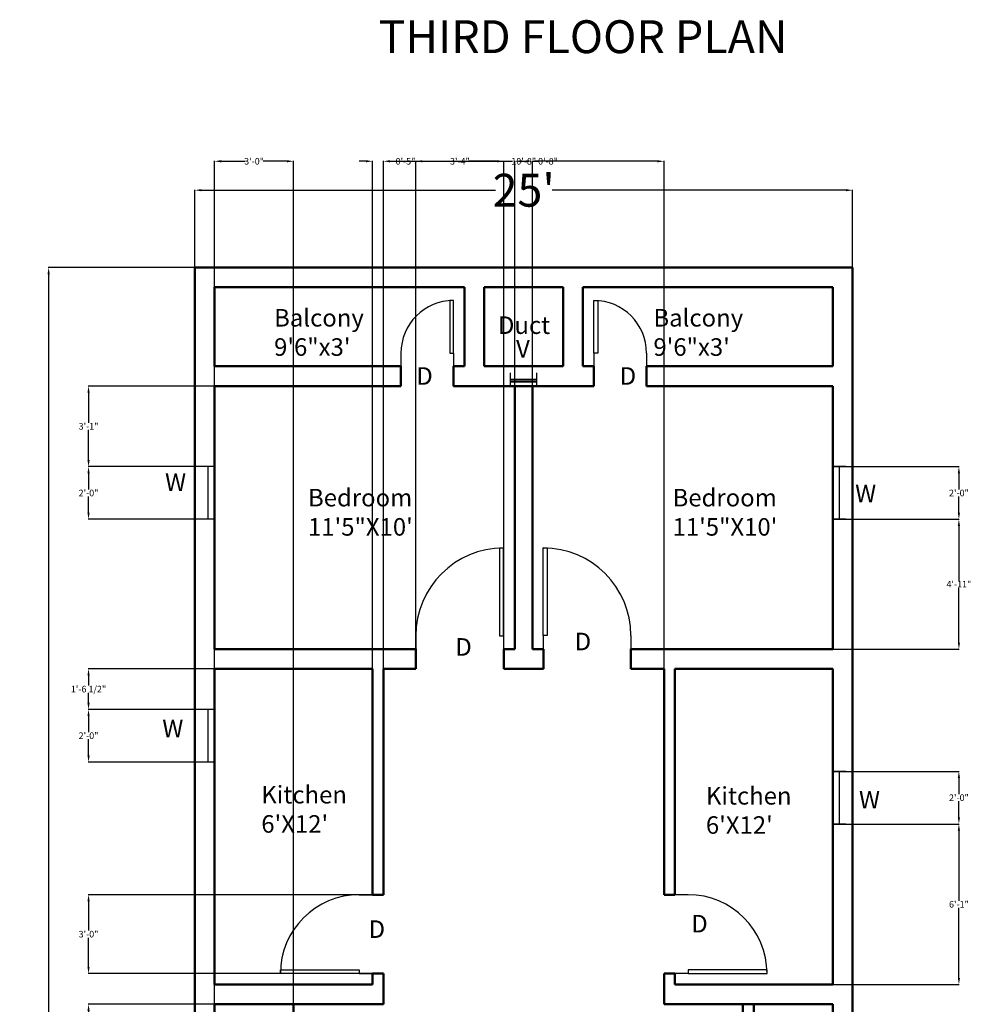
# Model space of a CAD drawing. Units: inches. Extents: x -250 to 2650, y 180 to 1183.
# Tile 8 of 10: x 1594 to 2028, y 734 to 1183. Entities that reach past the tile are written whole.
import ezdxf

# ---------------------------------------------------------------- set-up
doc = ezdxf.new("R2010")
doc.units = ezdxf.units.IN
doc.header["$MEASUREMENT"] = 0
for name, color, linetype, lineweight in [('A-ANNO-DIMS', 2, 'Continuous', 18), ('A-ANNO-TEXT', 7, 'Continuous', 18), ('A-AREA-IDEN', 3, 'Continuous', 18), ('A-DOOR', 4, 'Continuous', 25), ('A-GLAZ', 3, 'Continuous', 25), ('A-WALL', 7, 'Continuous', 50)]:
    doc.layers.add(name, color=color, linetype=linetype, lineweight=lineweight)
doc.styles.get("Standard").update_dxf_attribs({"font": 'arial.ttf'})
doc.dimstyles.get("Standard").update_dxf_attribs({"dimtxt": 3, "dimasz": 3, "dimexe": 0.18, "dimexo": 0.0625, "dimgap": 0.09, "dimtad": 0, "dimtih": 1, "dimtoh": 1, "dimdec": 0, "dimzin": 0, "dimdsep": 46, "dimlunit": 3, "dimtxsty": 'Standard', "dimcen": 0.09, "dimadec": 0, "dimazin": 0, "dimtfac": 1, "dimtdec": 0, "dimtofl": 0, "dimtmove": 0, "dimatfit": 3, "dimfxl": 1, "dimtolj": 1, "dimtzin": 0, "dimarcsym": 0})

# ---------------------------------------------------------------- blocks, each defined once
blk = doc.blocks.new('*D36')
at = {"layer": 'A-ANNO-DIMS', "color": 0, "lineweight": -2, "transparency": 16777216}
for p, q in [((1673.49, 1070.09), (1673.49, 1105.5)), ((1676.49, 1105.32), (1810.55, 1105.32)), ((1970.49, 1105.32), (1836.44, 1105.32)), ((1973.49, 1070.09), (1973.49, 1105.5))]:
    blk.add_line(p, q, dxfattribs=at)
at = {"layer": 'A-ANNO-DIMS', "color": 0, "transparency": 16777216}
for points in [[(1676.49, 1105.82), (1676.49, 1104.82), (1673.49, 1105.32)], [(1970.49, 1105.82), (1970.49, 1104.82), (1973.49, 1105.32)]]:
    blk.add_solid(points, dxfattribs=at)
at = {"layer": 'Defpoints', "color": 0, "transparency": 16777216}
for p in [(1673.49, 1105.32), (1673.49, 1070.02), (1973.49, 1070.02)]:
    blk.add_point(p, dxfattribs=at)
at = {"layer": 'A-ANNO-DIMS', "color": 0, "transparency": 16777216, "insert": (1823.49, 1105.32), "char_height": 3, "attachment_point": 5}
blk.add_mtext("\\A1;{\\H5x;25'}", dxfattribs=at)
blk = doc.blocks.new('*D37')
at = {"layer": 'A-ANNO-DIMS', "color": 0, "lineweight": -2, "transparency": 16777216}
for p, q in [((1673.43, 1070.02), (1606.61, 1070.02)), ((1606.79, 1067.02), (1606.79, 657.77)), ((1606.79, 233.02), (1606.79, 642.28)), ((1673.43, 230.02), (1606.61, 230.02))]:
    blk.add_line(p, q, dxfattribs=at)
at = {"layer": 'A-ANNO-DIMS', "color": 0, "transparency": 16777216}
for points in [[(1606.29, 1067.02), (1607.29, 1067.02), (1606.79, 1070.02)], [(1606.29, 233.02), (1607.29, 233.02), (1606.79, 230.02)]]:
    blk.add_solid(points, dxfattribs=at)
at = {"layer": 'Defpoints', "color": 0, "transparency": 16777216}
for p in [(1673.49, 1070.02), (1606.79, 230.02), (1673.49, 230.02)]:
    blk.add_point(p, dxfattribs=at)
at = {"layer": 'A-ANNO-DIMS', "color": 0, "transparency": 16777216, "insert": (1606.79, 650.02), "char_height": 3, "attachment_point": 5}
blk.add_mtext("\\A1;{\\H5x;70'}", dxfattribs=at)
blk = doc.blocks.new('*U17')
for p, q in [((-24, 0), (-24, -6)), ((0, 0), (0, -6))]:
    blk.add_line(p, q)
blk.add_lwpolyline([(0, 0), (0, 24), (-1.75, 24), (-1.75, 0)], close=True)
blk.add_arc((0, 0), 24, 90, 180)
blk = doc.blocks.new('*U18')
for p, q in [((0, 0), (0, -6)), ((24, 0), (24, -6))]:
    blk.add_line(p, q)
blk.add_lwpolyline([(0, 0), (0, 24), (1.75, 24), (1.75, 0)], close=True)
blk.add_arc((0, 0), 24, 0, 90)
blk = doc.blocks.new('*U24')
for p, q in [((-24, 6), (-24, 0)), ((0, 6), (0, 0)), ((0, 3), (-24, 3))]:
    blk.add_line(p, q)
blk = doc.blocks.new('*U23')
for p, q in [((-24, 6), (-24, 0)), ((0, 6), (0, 0)), ((0, 3), (-24, 3))]:
    blk.add_line(p, q)
blk = doc.blocks.new('*U40')
for p, q in [((0, 0), (0, -6)), ((40, 0), (40, -6))]:
    blk.add_line(p, q)
blk.add_lwpolyline([(0, 0), (0, 40), (1.75, 40), (1.75, 0)], close=True)
blk.add_arc((0, 0), 40, 0, 90)
blk = doc.blocks.new('*U41')
for p, q in [((0, 0), (0, -6)), ((-40, 0), (-40, -6))]:
    blk.add_line(p, q)
blk.add_lwpolyline([(0, 0), (0, 40), (-1.75, 40), (-1.75, 0)], close=True)
blk.add_arc((0, 0), 40, 90, 180)
blk = doc.blocks.new('*U42')
for p, q in [((0, 0), (0, -6)), ((-36, 0), (-36, -6))]:
    blk.add_line(p, q)
blk.add_lwpolyline([(0, 0), (0, 36), (-1.75, 36), (-1.75, 0)], close=True)
blk.add_arc((0, 0), 36, 90, 180)
blk = doc.blocks.new('*U43')
for p, q in [((-36, 0), (-36, 6)), ((0, 0), (0, 6))]:
    blk.add_line(p, q)
blk.add_lwpolyline([(0, 0), (0, -36), (-1.75, -36), (-1.75, 0)], close=True)
blk.add_arc((0, 0), 36, 180, 270)
blk = doc.blocks.new('*U22')
for p, q in [((0, 6), (0, 0)), ((12, 6), (12, 0)), ((0, 3), (12, 3))]:
    blk.add_line(p, q)
blk = doc.blocks.new('*D143')
at = {"layer": 'A-ANNO-DIMS', "color": 0, "lineweight": -2, "transparency": 16777216}
for p, q in [((1682.49, 734.09), (1682.49, 1118.7)), ((1685.49, 1118.52), (1696.42, 1118.52)), ((1715.49, 1118.52), (1704.57, 1118.52)), ((1718.49, 734.09), (1718.49, 1118.7))]:
    blk.add_line(p, q, dxfattribs=at)
at = {"layer": 'A-ANNO-DIMS', "color": 0, "transparency": 16777216}
for points in [[(1685.49, 1119.02), (1685.49, 1118.02), (1682.49, 1118.52)], [(1715.49, 1119.02), (1715.49, 1118.02), (1718.49, 1118.52)]]:
    blk.add_solid(points, dxfattribs=at)
at = {"layer": 'Defpoints', "color": 0, "transparency": 16777216}
for p in [(1718.49, 1118.52), (1682.49, 734.02), (1718.49, 734.02)]:
    blk.add_point(p, dxfattribs=at)
at = {"layer": 'A-ANNO-DIMS', "color": 0, "transparency": 16777216, "insert": (1700.49, 1118.52), "char_height": 3, "attachment_point": 5}
blk.add_mtext('\\A1;3\'-0"', dxfattribs=at)
blk = doc.blocks.new('*D145')
at = {"layer": 'A-ANNO-DIMS', "color": 0, "lineweight": -2, "transparency": 16777216}
for p, q in [((1682.43, 734.02), (1624.81, 734.02)), ((1624.99, 731.02), (1624.99, 717.09)), ((1624.99, 699.91), (1624.99, 713.84)), ((1682.43, 696.91), (1624.81, 696.91))]:
    blk.add_line(p, q, dxfattribs=at)
at = {"layer": 'A-ANNO-DIMS', "color": 0, "transparency": 16777216}
for points in [[(1624.49, 731.02), (1625.49, 731.02), (1624.99, 734.02)], [(1624.49, 699.91), (1625.49, 699.91), (1624.99, 696.91)]]:
    blk.add_solid(points, dxfattribs=at)
at = {"layer": 'Defpoints', "color": 0, "transparency": 16777216}
for p in [(1624.99, 734.02), (1682.49, 734.02), (1682.49, 696.91)]:
    blk.add_point(p, dxfattribs=at)
at = {"layer": 'A-ANNO-DIMS', "color": 0, "transparency": 16777216, "insert": (1624.99, 715.47), "char_height": 3, "attachment_point": 5}
blk.add_mtext('\\A1;3\'-1"', dxfattribs=at)
blk = doc.blocks.new('*D153')
at = {"layer": 'A-ANNO-DIMS', "color": 0, "lineweight": -2, "transparency": 16777216}
for p, q in [((1819.49, 1016.09), (1819.49, 1118.7)), ((1822.49, 1118.52), (1824.49, 1118.52)), ((1827.49, 1016.09), (1827.49, 1118.7)), ((1827.49, 1118.52), (1830.49, 1118.52))]:
    blk.add_line(p, q, dxfattribs=at)
at = {"layer": 'A-ANNO-DIMS', "color": 0, "transparency": 16777216}
for points in [[(1822.49, 1119.02), (1822.49, 1118.02), (1819.49, 1118.52)], [(1824.49, 1119.02), (1824.49, 1118.02), (1827.49, 1118.52)]]:
    blk.add_solid(points, dxfattribs=at)
at = {"layer": 'Defpoints', "color": 0, "transparency": 16777216}
for p in [(1827.49, 1118.52), (1819.49, 1016.02), (1827.49, 1016.02)]:
    blk.add_point(p, dxfattribs=at)
at = {"layer": 'A-ANNO-DIMS', "color": 0, "transparency": 16777216, "insert": (1834.57, 1118.52), "char_height": 3, "attachment_point": 5}
blk.add_mtext('\\A1;0\'-8"', dxfattribs=at)
blk = doc.blocks.new('*D154')
at = {"layer": 'A-ANNO-DIMS', "color": 0, "lineweight": -2, "transparency": 16777216}
for p, q in [((1774.26, 896.09), (1774.26, 1118.7)), ((1777.26, 1118.52), (1790.3, 1118.52)), ((1811.49, 1118.52), (1798.45, 1118.52)), ((1814.49, 896.09), (1814.49, 1118.7))]:
    blk.add_line(p, q, dxfattribs=at)
at = {"layer": 'A-ANNO-DIMS', "color": 0, "transparency": 16777216}
for points in [[(1777.26, 1119.02), (1777.26, 1118.02), (1774.26, 1118.52)], [(1811.49, 1119.02), (1811.49, 1118.02), (1814.49, 1118.52)]]:
    blk.add_solid(points, dxfattribs=at)
at = {"layer": 'Defpoints', "color": 0, "transparency": 16777216}
for p in [(1814.49, 1118.52), (1774.26, 896.02), (1814.49, 896.02)]:
    blk.add_point(p, dxfattribs=at)
at = {"layer": 'A-ANNO-DIMS', "color": 0, "transparency": 16777216, "insert": (1794.38, 1118.52), "char_height": 3, "attachment_point": 5}
blk.add_mtext('\\A1;3\'-4"', dxfattribs=at)
blk = doc.blocks.new('*D155')
at = {"layer": 'A-ANNO-DIMS', "color": 0, "lineweight": -2, "transparency": 16777216}
for p, q in [((1751.49, 1118.52), (1748.49, 1118.52)), ((1754.49, 887.09), (1754.49, 1118.7)), ((1759.49, 887.09), (1759.49, 1118.7)), ((1762.49, 1118.52), (1765.49, 1118.52))]:
    blk.add_line(p, q, dxfattribs=at)
at = {"layer": 'A-ANNO-DIMS', "color": 0, "transparency": 16777216}
for points in [[(1751.49, 1119.02), (1751.49, 1118.02), (1754.49, 1118.52)], [(1762.49, 1119.02), (1762.49, 1118.02), (1759.49, 1118.52)]]:
    blk.add_solid(points, dxfattribs=at)
at = {"layer": 'Defpoints', "color": 0, "transparency": 16777216}
for p in [(1759.49, 1118.52), (1754.49, 887.02), (1759.49, 887.02)]:
    blk.add_point(p, dxfattribs=at)
at = {"layer": 'A-ANNO-DIMS', "color": 0, "transparency": 16777216, "insert": (1769.57, 1118.52), "char_height": 3, "attachment_point": 5}
blk.add_mtext('\\A1;0\'-5"', dxfattribs=at)
blk = doc.blocks.new('*D156')
at = {"layer": 'A-ANNO-DIMS', "color": 0, "lineweight": -2, "transparency": 16777216}
for p, q in [((1759.49, 887.09), (1759.49, 1118.7)), ((1762.49, 1118.52), (1818.39, 1118.52)), ((1884.49, 1118.52), (1828.59, 1118.52)), ((1887.49, 887.09), (1887.49, 1118.7))]:
    blk.add_line(p, q, dxfattribs=at)
at = {"layer": 'A-ANNO-DIMS', "color": 0, "transparency": 16777216}
for points in [[(1762.49, 1119.02), (1762.49, 1118.02), (1759.49, 1118.52)], [(1884.49, 1119.02), (1884.49, 1118.02), (1887.49, 1118.52)]]:
    blk.add_solid(points, dxfattribs=at)
at = {"layer": 'Defpoints', "color": 0, "transparency": 16777216}
for p in [(1887.49, 1118.52), (1759.49, 887.02), (1887.49, 887.02)]:
    blk.add_point(p, dxfattribs=at)
at = {"layer": 'A-ANNO-DIMS', "color": 0, "transparency": 16777216, "insert": (1823.49, 1118.52), "char_height": 3, "attachment_point": 5}
blk.add_mtext('\\A1;10\'-8"', dxfattribs=at)
blk = doc.blocks.new('*D157')
at = {"layer": 'A-ANNO-DIMS', "color": 0, "lineweight": -2, "transparency": 16777216}
for p, q in [((1759.43, 784.02), (1624.81, 784.02)), ((1624.99, 781.02), (1624.99, 767.65)), ((1624.99, 751.02), (1624.99, 764.4)), ((1759.43, 748.02), (1624.81, 748.02))]:
    blk.add_line(p, q, dxfattribs=at)
at = {"layer": 'A-ANNO-DIMS', "color": 0, "transparency": 16777216}
for points in [[(1624.49, 781.02), (1625.49, 781.02), (1624.99, 784.02)], [(1624.49, 751.02), (1625.49, 751.02), (1624.99, 748.02)]]:
    blk.add_solid(points, dxfattribs=at)
at = {"layer": 'Defpoints', "color": 0, "transparency": 16777216}
for p in [(1624.99, 784.02), (1759.49, 784.02), (1759.49, 748.02)]:
    blk.add_point(p, dxfattribs=at)
at = {"layer": 'A-ANNO-DIMS', "color": 0, "transparency": 16777216, "insert": (1624.99, 766.02), "char_height": 3, "attachment_point": 5}
blk.add_mtext('\\A1;3\'-0"', dxfattribs=at)
blk = doc.blocks.new('*D158')
at = {"layer": 'A-ANNO-DIMS', "color": 0, "lineweight": -2, "transparency": 16777216}
for p, q in [((1682.43, 979.23), (1624.81, 979.23)), ((1624.99, 976.23), (1624.99, 968.85)), ((1624.99, 958.23), (1624.99, 965.61)), ((1682.43, 955.23), (1624.81, 955.23))]:
    blk.add_line(p, q, dxfattribs=at)
at = {"layer": 'A-ANNO-DIMS', "color": 0, "transparency": 16777216}
for points in [[(1624.49, 976.23), (1625.49, 976.23), (1624.99, 979.23)], [(1624.49, 958.23), (1625.49, 958.23), (1624.99, 955.23)]]:
    blk.add_solid(points, dxfattribs=at)
at = {"layer": 'Defpoints', "color": 0, "transparency": 16777216}
for p in [(1624.99, 979.23), (1682.49, 979.23), (1682.49, 955.23)]:
    blk.add_point(p, dxfattribs=at)
at = {"layer": 'A-ANNO-DIMS', "color": 0, "transparency": 16777216, "insert": (1624.99, 967.23), "char_height": 3, "attachment_point": 5}
blk.add_mtext('\\A1;2\'-0"', dxfattribs=at)
blk = doc.blocks.new('*D159')
at = {"layer": 'A-ANNO-DIMS', "color": 0, "lineweight": -2, "transparency": 16777216}
for p, q in [((1682.43, 1016.02), (1624.81, 1016.02)), ((1624.99, 1013.02), (1624.99, 999.25)), ((1624.99, 982.23), (1624.99, 996.01)), ((1682.43, 979.23), (1624.81, 979.23))]:
    blk.add_line(p, q, dxfattribs=at)
at = {"layer": 'A-ANNO-DIMS', "color": 0, "transparency": 16777216}
for points in [[(1624.49, 1013.02), (1625.49, 1013.02), (1624.99, 1016.02)], [(1624.49, 982.23), (1625.49, 982.23), (1624.99, 979.23)]]:
    blk.add_solid(points, dxfattribs=at)
at = {"layer": 'Defpoints', "color": 0, "transparency": 16777216}
for p in [(1624.99, 1016.02), (1682.49, 1016.02), (1682.49, 979.23)]:
    blk.add_point(p, dxfattribs=at)
at = {"layer": 'A-ANNO-DIMS', "color": 0, "transparency": 16777216, "insert": (1624.99, 997.63), "char_height": 3, "attachment_point": 5}
blk.add_mtext('\\A1;3\'-1"', dxfattribs=at)
blk = doc.blocks.new('*D160')
at = {"layer": 'A-ANNO-DIMS', "color": 0, "lineweight": -2, "transparency": 16777216}
for p, q in [((1682.43, 868.53), (1624.81, 868.53)), ((1624.99, 865.53), (1624.99, 858.15)), ((1624.99, 847.53), (1624.99, 854.91)), ((1682.43, 844.53), (1624.81, 844.53))]:
    blk.add_line(p, q, dxfattribs=at)
at = {"layer": 'A-ANNO-DIMS', "color": 0, "transparency": 16777216}
for points in [[(1624.49, 865.53), (1625.49, 865.53), (1624.99, 868.53)], [(1624.49, 847.53), (1625.49, 847.53), (1624.99, 844.53)]]:
    blk.add_solid(points, dxfattribs=at)
at = {"layer": 'Defpoints', "color": 0, "transparency": 16777216}
for p in [(1624.99, 868.53), (1682.49, 868.53), (1682.49, 844.53)]:
    blk.add_point(p, dxfattribs=at)
at = {"layer": 'A-ANNO-DIMS', "color": 0, "transparency": 16777216, "insert": (1624.99, 856.53), "char_height": 3, "attachment_point": 5}
blk.add_mtext('\\A1;2\'-0"', dxfattribs=at)
blk = doc.blocks.new('*D161')
at = {"layer": 'A-ANNO-DIMS', "color": 0, "lineweight": -2, "transparency": 16777216}
for p, q in [((1682.43, 887.02), (1624.81, 887.02)), ((1624.99, 884.02), (1624.99, 879.42)), ((1624.99, 871.53), (1624.99, 876.14)), ((1682.43, 868.53), (1624.81, 868.53))]:
    blk.add_line(p, q, dxfattribs=at)
at = {"layer": 'A-ANNO-DIMS', "color": 0, "transparency": 16777216}
for points in [[(1624.49, 884.02), (1625.49, 884.02), (1624.99, 887.02)], [(1624.49, 871.53), (1625.49, 871.53), (1624.99, 868.53)]]:
    blk.add_solid(points, dxfattribs=at)
at = {"layer": 'Defpoints', "color": 0, "transparency": 16777216}
for p in [(1624.99, 887.02), (1682.49, 887.02), (1682.49, 868.53)]:
    blk.add_point(p, dxfattribs=at)
at = {"layer": 'A-ANNO-DIMS', "color": 0, "transparency": 16777216, "insert": (1624.99, 877.78), "char_height": 3, "attachment_point": 5}
blk.add_mtext('\\A1;1\'-6 1/2"', dxfattribs=at)
blk = doc.blocks.new('*D162')
at = {"layer": 'A-ANNO-DIMS', "color": 0, "lineweight": -2, "transparency": 16777216}
for p, q in [((1964.55, 979.23), (2022.17, 979.23)), ((2021.99, 976.23), (2021.99, 968.85)), ((2021.99, 958.23), (2021.99, 965.61)), ((1964.55, 955.23), (2022.17, 955.23))]:
    blk.add_line(p, q, dxfattribs=at)
at = {"layer": 'A-ANNO-DIMS', "color": 0, "transparency": 16777216}
for points in [[(2021.49, 976.23), (2022.49, 976.23), (2021.99, 979.23)], [(2021.49, 958.23), (2022.49, 958.23), (2021.99, 955.23)]]:
    blk.add_solid(points, dxfattribs=at)
at = {"layer": 'Defpoints', "color": 0, "transparency": 16777216}
for p in [(1964.49, 979.23), (2021.99, 979.23), (1964.49, 955.23)]:
    blk.add_point(p, dxfattribs=at)
at = {"layer": 'A-ANNO-DIMS', "color": 0, "transparency": 16777216, "insert": (2021.99, 967.23), "char_height": 3, "attachment_point": 5}
blk.add_mtext('\\A1;2\'-0"', dxfattribs=at)
blk = doc.blocks.new('*D163')
at = {"layer": 'A-ANNO-DIMS', "color": 0, "lineweight": -2, "transparency": 16777216}
for p, q in [((1964.55, 955.23), (2022.17, 955.23)), ((2021.99, 952.23), (2021.99, 927.22)), ((2021.99, 899.02), (2021.99, 924.03)), ((1964.55, 896.02), (2022.17, 896.02))]:
    blk.add_line(p, q, dxfattribs=at)
at = {"layer": 'A-ANNO-DIMS', "color": 0, "transparency": 16777216}
for points in [[(2021.49, 952.23), (2022.49, 952.23), (2021.99, 955.23)], [(2021.49, 899.02), (2022.49, 899.02), (2021.99, 896.02)]]:
    blk.add_solid(points, dxfattribs=at)
at = {"layer": 'Defpoints', "color": 0, "transparency": 16777216}
for p in [(1964.49, 955.23), (2021.99, 955.23), (1964.49, 896.02)]:
    blk.add_point(p, dxfattribs=at)
at = {"layer": 'A-ANNO-DIMS', "color": 0, "transparency": 16777216, "insert": (2021.99, 925.63), "char_height": 3, "attachment_point": 5}
blk.add_mtext('\\A1;4\'-11"', dxfattribs=at)
blk = doc.blocks.new('*D164')
at = {"layer": 'A-ANNO-DIMS', "color": 0, "lineweight": -2, "transparency": 16777216}
for p, q in [((1964.55, 840.25), (2022.17, 840.25)), ((2021.99, 837.25), (2021.99, 829.87)), ((2021.99, 819.25), (2021.99, 826.63)), ((1964.55, 816.25), (2022.17, 816.25))]:
    blk.add_line(p, q, dxfattribs=at)
at = {"layer": 'A-ANNO-DIMS', "color": 0, "transparency": 16777216}
for points in [[(2021.49, 837.25), (2022.49, 837.25), (2021.99, 840.25)], [(2021.49, 819.25), (2022.49, 819.25), (2021.99, 816.25)]]:
    blk.add_solid(points, dxfattribs=at)
at = {"layer": 'Defpoints', "color": 0, "transparency": 16777216}
for p in [(1964.49, 840.25), (2021.99, 840.25), (1964.49, 816.25)]:
    blk.add_point(p, dxfattribs=at)
at = {"layer": 'A-ANNO-DIMS', "color": 0, "transparency": 16777216, "insert": (2021.99, 828.25), "char_height": 3, "attachment_point": 5}
blk.add_mtext('\\A1;2\'-0"', dxfattribs=at)
blk = doc.blocks.new('*D165')
at = {"layer": 'A-ANNO-DIMS', "color": 0, "lineweight": -2, "transparency": 16777216}
for p, q in [((1964.55, 816.25), (2022.17, 816.25)), ((2021.99, 813.25), (2021.99, 781.26)), ((2021.99, 746.02), (2021.99, 778.01)), ((1964.55, 743.02), (2022.17, 743.02))]:
    blk.add_line(p, q, dxfattribs=at)
at = {"layer": 'A-ANNO-DIMS', "color": 0, "transparency": 16777216}
for points in [[(2021.49, 813.25), (2022.49, 813.25), (2021.99, 816.25)], [(2021.49, 746.02), (2022.49, 746.02), (2021.99, 743.02)]]:
    blk.add_solid(points, dxfattribs=at)
at = {"layer": 'Defpoints', "color": 0, "transparency": 16777216}
for p in [(1964.49, 816.25), (2021.99, 816.25), (1964.49, 743.02)]:
    blk.add_point(p, dxfattribs=at)
at = {"layer": 'A-ANNO-DIMS', "color": 0, "transparency": 16777216, "insert": (2021.99, 779.64), "char_height": 3, "attachment_point": 5}
blk.add_mtext('\\A1;6\'-1"', dxfattribs=at)

msp = doc.modelspace()

# ---------------------------------------------------------------- linework, layer by layer
at = {"layer": 'A-WALL'}
for p, q in [((1973.49, 1070.02), (1673.49, 1070.02)), ((1673.49, 1070.02), (1673.49, 230.02)), ((1973.49, 230.02), (1973.49, 1070.02)), ((1796.49, 1061.02), (1682.49, 1061.02)), ((1682.49, 1061.02), (1682.49, 1025.02)), ((1796.49, 1061.02), (1796.49, 1025.02)), ((1841.49, 1061.02), (1805.49, 1061.02)), ((1805.49, 1061.02), (1805.49, 1025.02)), ((1841.49, 1025.02), (1841.49, 1061.02)), ((1850.49, 1025.02), (1850.49, 1061.02)), ((1964.49, 1061.02), (1850.49, 1061.02)), ((1964.49, 1025.02), (1964.49, 1061.02)), ((1964.49, 1025.02), (1964.49, 1061.02)), ((1964.49, 1025.02), (1964.49, 1061.02)), ((1964.49, 1025.02), (1964.49, 1061.02)), ((1767.49, 1025.02), (1682.49, 1025.02)), ((1767.49, 1025.02), (1767.49, 1016.02)), ((1796.49, 1025.02), (1791.49, 1025.02)), ((1791.49, 1016.02), (1791.49, 1025.02)), ((1841.49, 1025.02), (1805.49, 1025.02)), ((1855.49, 1025.02), (1850.49, 1025.02)), ((1855.49, 1016.02), (1855.49, 1025.02)), ((1964.49, 1025.02), (1879.49, 1025.02)), ((1879.49, 1025.02), (1879.49, 1016.02)), ((1767.49, 1016.02), (1682.49, 1016.02)), ((1682.49, 1016.02), (1682.49, 896.02)), ((1767.49, 1016.02), (1763.49, 1016.02)), ((1855.49, 1016.02), (1791.49, 1016.02)), ((1855.49, 1016.02), (1791.49, 1016.02)), ((1829.49, 1018.1), (1817.49, 1018.1)), ((1819.49, 1016.02), (1819.49, 896.02)), ((1827.49, 896.02), (1827.49, 1016.02)), ((1855.49, 1016.02), (1846.49, 1016.02)), ((1883.49, 1016.02), (1879.49, 1016.02)), ((1964.49, 1016.02), (1880.34, 1016.02)), ((1964.49, 896.02), (1964.49, 1016.02)), ((1964.49, 896.02), (1964.49, 1016.02)), ((1964.49, 896.02), (1964.49, 1016.02)), ((1774.26, 896.02), (1682.49, 896.02)), ((1774.26, 896.13), (1774.26, 887.02)), ((1819.49, 896.02), (1814.49, 896.02)), ((1814.49, 896.02), (1814.49, 887.02)), ((1832.49, 896.02), (1827.49, 896.02)), ((1832.49, 896.02), (1832.49, 887.02)), ((1872.38, 896.17), (1872.38, 887.02)), ((1887.49, 896.02), (1872.38, 896.02)), ((1964.49, 896.02), (1887.49, 896.02)), ((1682.49, 887.02), (1682.49, 743.02)), ((1754.49, 887.02), (1682.49, 887.02)), ((1754.49, 887.02), (1754.49, 784.02)), ((1759.49, 887.02), (1759.49, 784.02)), ((1774.26, 887.02), (1759.49, 887.02)), ((1832.49, 887.02), (1814.49, 887.02)), ((1887.49, 887.02), (1872.38, 887.02)), ((1887.49, 784.02), (1887.49, 887.02)), ((1964.49, 887.02), (1892.49, 887.02)), ((1964.49, 887.02), (1892.49, 887.02)), ((1892.49, 784.02), (1892.49, 887.02)), ((1964.49, 743.02), (1964.49, 887.02)), ((1964.49, 743.02), (1964.49, 887.02)), ((1964.49, 743.02), (1964.49, 887.02)), ((1754.49, 784.02), (1759.49, 784.02)), ((1892.49, 784.02), (1887.49, 784.02)), ((1754.49, 748.02), (1759.49, 748.02)), ((1754.49, 748.02), (1754.49, 743.02)), ((1759.49, 748.02), (1759.49, 734.02)), ((1887.49, 734.02), (1887.49, 748.02)), ((1892.49, 748.02), (1887.49, 748.02)), ((1892.49, 743.02), (1892.49, 748.02)), ((1754.49, 743.02), (1682.49, 743.02)), ((1964.49, 743.02), (1892.49, 743.02)), ((1759.49, 734.02), (1682.49, 734.02)), ((1682.49, 734.02), (1682.49, 696.91)), ((1718.49, 696.91), (1718.49, 734.02)), ((1964.49, 734.02), (1887.49, 734.02)), ((1923.49, 686.91), (1923.49, 734.02)), ((1923.49, 686.91), (1923.49, 734.02)), ((1928.49, 696.91), (1928.49, 734.02)), ((1964.49, 696.91), (1964.49, 734.02)), ((1964.49, 716.02), (1964.49, 734.02))]:
    msp.add_line(p, q, dxfattribs=at)

# ---------------------------------------------------------------- block references
at = {"layer": 'A-DOOR'}
for name, p in [('*U17', (1791.49, 1031.02)), ('*U18', (1855.49, 1031.02)), ('*U41', (1814.26, 902.13)), ('*U40', (1832.38, 902.17))]:
    msp.add_blockref(name, p, dxfattribs=at)
at = {"layer": 'A-DOOR', "rotation": 270}
for name, p in [('*U43', (1748.49, 748.02)), ('*U42', (1898.49, 748.02))]:
    msp.add_blockref(name, p, dxfattribs=at)
at = {"layer": 'A-GLAZ'}
for name, p, rotation in [('*U22', (1829.49, 1022.02), 180), ('*U23', (1676.49, 955.23), 270), ('*U24', (1964.49, 955.23), 270), ('*U23', (1676.49, 844.53), 270), ('*U24', (1964.49, 816.25), 270)]:
    msp.add_blockref(name, p, dxfattribs=dict(at, rotation=rotation))

# ---------------------------------------------------------------- texts
at = {"layer": 'A-ANNO-TEXT', "attachment_point": 1}
for s, width, insert, char_height in [('THIRD FLOOR PLAN ', 207.4062, (1757.3, 1182.82), 15), ('V', 10.3916, (1820, 1036.98), 8), ('D', 10.3916, (1774.48, 1024.6), 8), ('D', 10.3916, (1867.28, 1024.6), 8), ('W', 10.3916, (1659.91, 976.14), 8), ('W', 10.3916, (1974.67, 971.03), 8), ('D', 10.3916, (1846.73, 903.49), 8), ('D', 10.3916, (1792.29, 901.02), 8), ('W', 10.3916, (1658.64, 863.8), 8), ('W', 10.3916, (1976.41, 831.35), 8), ('D', 10.3916, (1899.91, 774.79), 8), ('D', 10.3916, (1752.74, 772.3), 8)]:
    msp.add_mtext_dynamic_manual_height_columns(s, width=width, gutter_width=1, heights=[0], dxfattribs=dict(at, insert=insert, char_height=char_height))
at = {"layer": 'A-AREA-IDEN', "attachment_point": 1}
for s, width, heights, insert, char_height in [('Balcony 9\'6"x3\'', 37.1044, [0], (1709.63, 1051.13), 8), ('Balcony 9\'6"x3\'', 37.1044, [0], (1882.65, 1051.13), 8), ('{\\H2.66667x;Duct} ', 7.71, [3.05], (1811.74, 1047.76), 3), ('Bedroom \\P11\'5"X10\'', 51.3886, [0], (1725.1, 969.1), 8), ('Bedroom \\P11\'5"X10\'', 51.3886, [0], (1891.39, 969.1), 8), ("Kitchen 6'X12'", 37.1044, [0], (1703.79, 833.62), 8), ("Kitchen 6'X12'", 37.1044, [0], (1906.58, 833.12), 8)]:
    msp.add_mtext_dynamic_manual_height_columns(s, width=width, gutter_width=1, heights=heights, dxfattribs=dict(at, insert=insert, char_height=char_height))

# ---------------------------------------------------------------- dimensions: what is measured, and where the dimension line sits
at = {"layer": 'A-ANNO-DIMS'}
for base, p1, p2, picture, middle in [((1718.49, 1118.52), (1682.49, 734.02), (1718.49, 734.02), '*D143', (1700.49, 1118.52)), ((1759.49, 1118.52), (1754.49, 887.02), (1759.49, 887.02), '*D155', (1769.57, 1118.52)), ((1887.49, 1118.52), (1759.49, 887.02), (1887.49, 887.02), '*D156', (1823.49, 1118.52)), ((1814.49, 1118.52), (1774.26, 896.02), (1814.49, 896.02), '*D154', (1794.38, 1118.52)), ((1827.49, 1118.52), (1819.49, 1016.02), (1827.49, 1016.02), '*D153', (1834.57, 1118.52))]:
    dim = msp.add_linear_dim(base=base, p1=p1, p2=p2, dimstyle='Standard', override={"dimdec": 1, "dimlfac": 1, "dimrnd": 0, "dimzin": 1, "dimdsep": 46, "dimlunit": 4, "dimfrac": 2}, dxfattribs=at)
    dim.commit()
    dim.dimension.update_dxf_attribs({"geometry": picture, "text_midpoint": middle})
dim = msp.add_linear_dim(base=(1673.49, 1105.32), p1=(1973.49, 1070.02), p2=(1673.49, 1070.02), text='{\\H5x;<>}', dimstyle='Standard', override={"dimclrd": 0, "dimclre": 0, "dimclrt": 0}, dxfattribs=at)
dim.commit()
dim.dimension.update_dxf_attribs({"geometry": '*D36', "text_midpoint": (1823.49, 1105.32)})
dim = msp.add_linear_dim(base=(1606.79, 230.02), p1=(1673.49, 1070.02), p2=(1673.49, 230.02), angle=90, text='{\\H5x;<>}', dimstyle='Standard', override={"dimclrd": 0, "dimclre": 0, "dimclrt": 0}, dxfattribs=at)
dim.commit()
dim.dimension.update_dxf_attribs({"geometry": '*D37', "text_midpoint": (1606.79, 650.02)})
for base, p1, p2, picture, middle in [((1624.99, 1016.02), (1682.49, 979.23), (1682.49, 1016.02), '*D159', (1624.99, 997.63)), ((1624.99, 979.23), (1682.49, 955.23), (1682.49, 979.23), '*D158', (1624.99, 967.23)), ((2021.99, 979.23), (1964.49, 955.23), (1964.49, 979.23), '*D162', (2021.99, 967.23)), ((2021.99, 955.23), (1964.49, 896.02), (1964.49, 955.23), '*D163', (2021.99, 925.63)), ((1624.99, 887.02), (1682.49, 868.53), (1682.49, 887.02), '*D161', (1624.99, 877.78)), ((1624.99, 868.53), (1682.49, 844.53), (1682.49, 868.53), '*D160', (1624.99, 856.53)), ((2021.99, 840.25), (1964.49, 816.25), (1964.49, 840.25), '*D164', (2021.99, 828.25)), ((2021.99, 816.25), (1964.49, 743.02), (1964.49, 816.25), '*D165', (2021.99, 779.64)), ((1624.99, 784.02), (1759.49, 748.02), (1759.49, 784.02), '*D157', (1624.99, 766.02)), ((1624.99, 734.02), (1682.49, 696.91), (1682.49, 734.02), '*D145', (1624.99, 715.47))]:
    dim = msp.add_linear_dim(base=base, p1=p1, p2=p2, angle=90, dimstyle='Standard', override={"dimdec": 1, "dimlfac": 1, "dimrnd": 0, "dimzin": 1, "dimdsep": 46, "dimlunit": 4, "dimfrac": 2}, dxfattribs=at)
    dim.commit()
    dim.dimension.update_dxf_attribs({"geometry": picture, "text_midpoint": middle})

doc.saveas('drawing.dxf')
